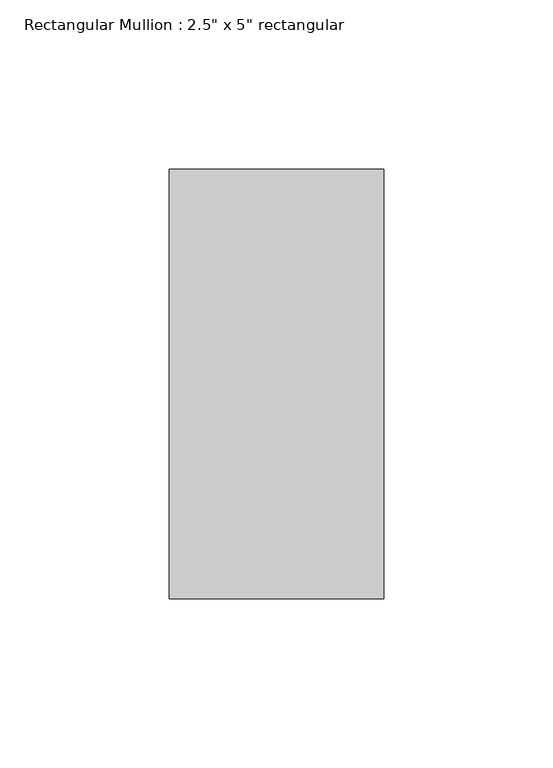
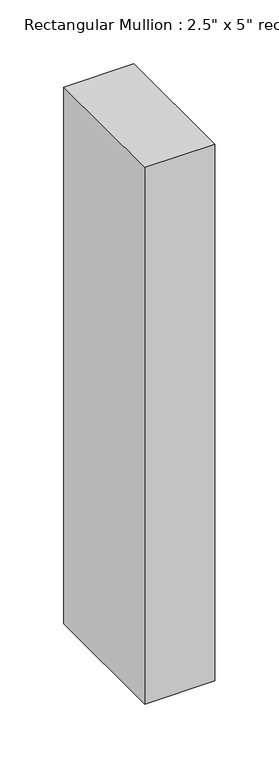
"""IFC4 building model written with IfcOpenShell, lengths in millimetres: member geometry."""

from ifc_helpers import new_model, si_unit, frame, origin, place, context, project, spatial, polyline, outline, extrude, source, transform, mapped, element, save


def member_794f270d(model_context):
    return source(origin(), model_context, "Body", "SweptSolid", [
        extrude(outline(polyline([(0.0, 63.5), (0.0, -63.5), (-63.5, -63.5), (-63.5, 63.5), (0.0, 63.5)])), frame((0.0, 0.0, -513.6068067), z_axis=(0.0, 0.0, 1.0), x_axis=(1.0, 0.0, 0.0)), (0.0, 0.0, 1.0), 513.6068067),
    ])


if __name__ == "__main__":
    model = new_model("IFC4")
    model_context = context("Model", 3, world=origin())
    ifc_project = project(units=[si_unit("LENGTHUNIT", "METRE", prefix="MILLI")], contexts=[model_context])
    site = spatial("IfcSite", under=ifc_project)
    building = spatial("IfcBuilding", under=site)
    placement = place(None, origin())
    member_shape = member_794f270d(model_context)
    element("IfcMember", 1, ObjectType="Rectangular Mullion : 2.5\" x 5\" rectangular", at=placement, inside=building, context=model_context, shape_type="MappedRepresentation", body=[
        mapped(member_shape, transform((0.0, 0.0, 0.0), x_axis=(1.0, 0.0, 0.0), y_axis=(0.0, 1.0, 0.0), z_axis=(0.0, 0.0, 1.0))),
    ])
    save(model, "model.ifc")

# Revit data of these elements
# Type "Rectangular Mullion : 2.5\" x 5\" rectangular"
#   built-in parameter 1007304 = 0.416667 (stored number, unit not read)
#   built-in parameter 1007301 = 0.104167 (stored number, unit not read)
#   built-in parameter 1007300 = 0.104167 (stored number, unit not read)
# Element 1 (IfcMember, "Rectangular Mullion : 2.5\" x 5\" rectangular")
#   Materials on its faces: "Aluminum"
# Materials
#   "Aluminum": class "Metal", colour RGB 247 247 247, transparency 0, Description = "Aluminum 6061", Cost = 0
